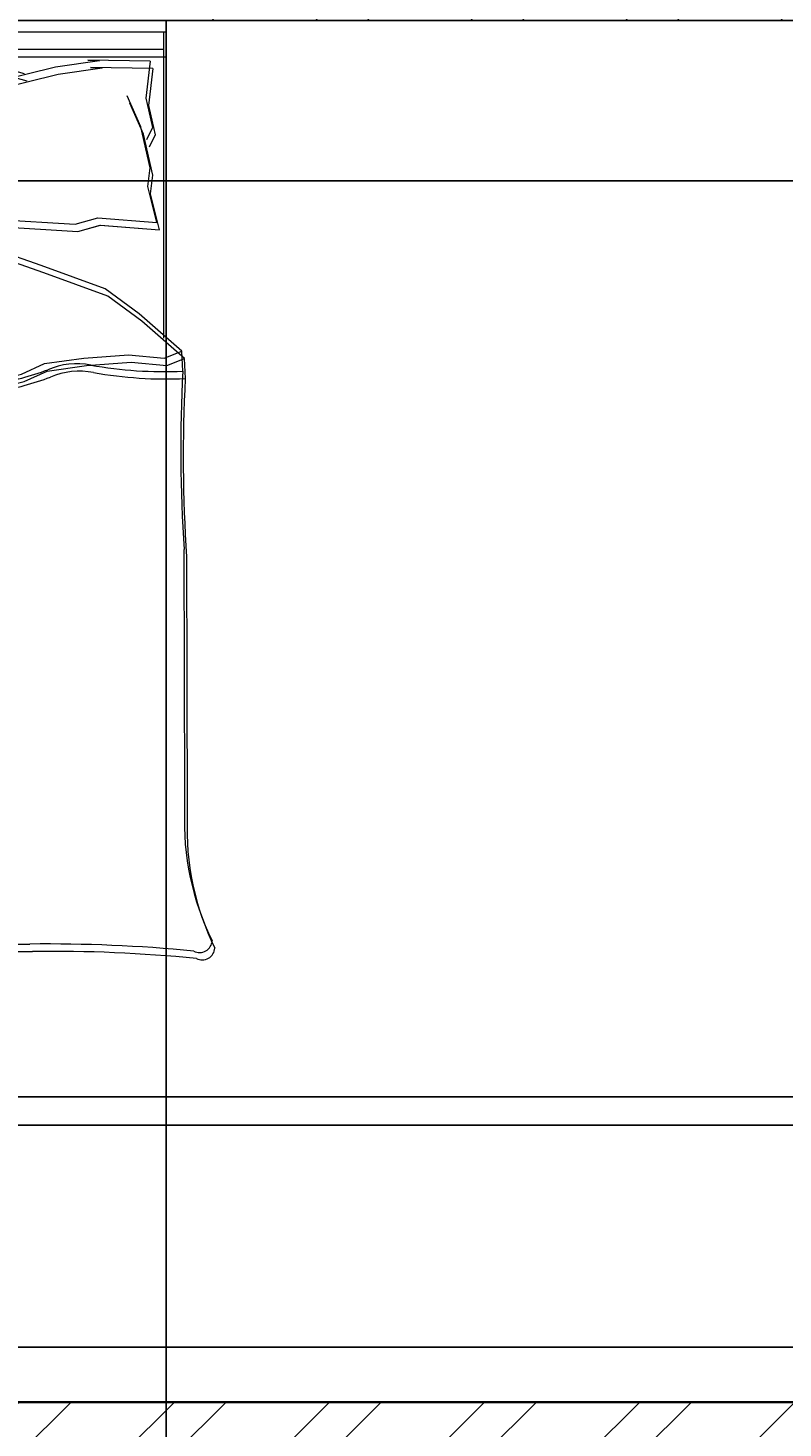
# Model space of a CAD drawing. Units: inches. Extents: x 1748 to 2382, y 1346 to 2284.
# Tile 22 of 26: x 1956 to 2022, y 2102 to 2223. Entities that reach past the tile are written whole.
import ezdxf

# ---------------------------------------------------------------- set-up
doc = ezdxf.new("R2010")
doc.units = ezdxf.units.IN
for name, color, linetype, lineweight in [('A-ANNO-DIMS', 2, 'Continuous', 18), ('A-FURN', 8, 'Continuous', 13), ('A-WALL', 7, 'Continuous', 35), ('A-WALL-PATT', 9, 'Continuous', 13)]:
    doc.layers.add(name, color=color, linetype=linetype, lineweight=lineweight)
doc.styles.get("Standard").update_dxf_attribs({"font": 'arial.ttf'})
doc.dimstyles.get("Standard").update_dxf_attribs({"dimtxt": 0.18, "dimasz": 0.18, "dimexe": 0.18, "dimexo": 0.0625, "dimgap": 0.09, "dimtad": 0, "dimtih": 1, "dimtoh": 1, "dimdec": 4, "dimzin": 0, "dimdsep": 46, "dimtxsty": 'Standard', "dimcen": 0.09, "dimadec": 0, "dimazin": 0, "dimtfac": 1, "dimtdec": 4, "dimtofl": 0, "dimtmove": 0, "dimatfit": 3, "dimfxl": 1, "dimtolj": 1, "dimtzin": 0, "dimarcsym": 0})

# ---------------------------------------------------------------- blocks, each defined once
blk = doc.blocks.new('BED-DOUBLE')
for p, q in [((3.48, 63.33), (3.48, 81.44)), ((3.48, 63.33), (3.48, 81.44)), ((3.48, 81.44), (51.49, 81.44)), ((3.7, 62.69), (3.7, 80.8)), ((3.7, 62.69), (3.7, 80.8)), ((51.27, 81.44), (51.27, 54.83)), ((51.27, 81.44), (51.27, 54.83)), ((51.49, 81.44), (51.49, 80.8)), ((51.49, 80.8), (51.49, 54.19)), ((51.49, 80.8), (51.49, 54.19)), ((3.48, 79.91), (51.27, 79.91)), ((3.48, 79.91), (51.27, 79.91)), ((3.7, 79.27), (51.49, 79.27)), ((3.7, 79.27), (51.49, 79.27)), ((16.88, 78.42), (19.77, 79.14)), ((16.88, 78.42), (19.77, 79.14)), ((19.77, 79.14), (20.09, 79.14)), ((19.77, 79.14), (20.09, 79.14)), ((20.09, 79.14), (24.54, 78.99)), ((20.09, 79.14), (24.54, 78.99)), ((24.54, 78.99), (25.98, 79.57)), ((24.54, 78.99), (25.98, 79.57)), ((25.98, 79.57), (26.56, 74.22)), ((25.98, 79.57), (26.56, 74.22)), ((3.89, 78.13), (4.47, 74.95)), ((3.9, 78.11), (8.18, 78.43)), ((3.9, 78.11), (8.18, 78.43)), ((3.9, 78.13), (4.47, 74.95)), ((8.18, 78.43), (8.29, 78.42)), ((8.18, 78.43), (8.28, 78.42)), ((8.28, 78.42), (12.11, 78.13)), ((8.29, 78.42), (12.11, 78.13)), ((12.11, 78.13), (17.6, 77.12)), ((12.11, 78.13), (17.6, 77.12)), ((14.86, 77.69), (16.88, 78.42)), ((14.86, 77.69), (16.88, 78.42)), ((17.11, 77.78), (20, 78.5)), ((17.11, 77.78), (20, 78.5)), ((20, 78.5), (20.32, 78.5)), ((20, 78.5), (20.32, 78.5)), ((20.32, 78.5), (24.77, 78.36)), ((20.32, 78.5), (24.77, 78.36)), ((24.77, 78.36), (26.21, 78.93)), ((24.77, 78.36), (26.21, 78.93)), ((26.21, 78.93), (26.79, 73.58)), ((26.21, 78.93), (26.79, 73.58)), ((27.98, 78.95), (27.73, 73.58)), ((27.98, 78.95), (27.73, 73.58)), ((28.21, 78.31), (27.96, 72.94)), ((28.21, 78.31), (27.96, 72.94)), ((29.46, 78.46), (27.98, 78.95)), ((29.46, 78.46), (27.98, 78.95)), ((29.68, 77.83), (28.21, 78.31)), ((29.68, 77.83), (28.21, 78.31)), ((33.88, 78.89), (29.46, 78.46)), ((33.88, 78.89), (29.46, 78.46)), ((34.11, 78.25), (29.68, 77.83)), ((34.11, 78.25), (29.68, 77.83)), ((34.21, 78.91), (33.88, 78.89)), ((34.2, 78.91), (33.88, 78.89)), ((34.43, 78.27), (34.11, 78.25)), ((34.43, 78.27), (34.11, 78.25)), ((37.14, 78.37), (34.2, 78.91)), ((37.14, 78.37), (34.21, 78.91)), ((37.36, 77.73), (34.43, 78.27)), ((37.36, 77.73), (34.43, 78.27)), ((41.91, 78.37), (36.5, 77.02)), ((41.91, 78.37), (36.5, 77.02)), ((39.2, 77.77), (37.14, 78.37)), ((39.2, 77.77), (37.14, 78.37)), ((45.71, 78.9), (41.91, 78.37)), ((45.71, 78.9), (41.91, 78.37)), ((45.94, 78.26), (42.14, 77.73)), ((45.94, 78.26), (42.14, 77.73)), ((50.11, 78.89), (44.71, 78.98)), ((44.71, 78.98), (45.71, 78.9)), ((50.11, 78.89), (44.71, 78.98)), ((44.71, 78.98), (45.71, 78.9)), ((50.34, 78.25), (44.94, 78.34)), ((44.94, 78.34), (45.94, 78.26)), ((50.34, 78.25), (44.94, 78.34)), ((44.94, 78.34), (45.94, 78.26)), ((50.11, 78.89), (49.73, 75.68)), ((50.11, 78.89), (49.73, 75.68)), ((50.34, 78.25), (49.96, 75.04)), ((50.34, 78.25), (49.96, 75.04)), ((4.12, 77.49), (4.7, 74.31)), ((4.12, 77.49), (4.7, 74.31)), ((4.13, 77.47), (8.41, 77.8)), ((4.13, 77.47), (8.41, 77.8)), ((8.41, 77.8), (8.51, 77.78)), ((8.41, 77.8), (8.51, 77.78)), ((8.51, 77.78), (12.34, 77.49)), ((8.51, 77.78), (12.34, 77.49)), ((12.34, 77.49), (17.83, 76.48)), ((12.34, 77.49), (17.83, 76.48)), ((15.08, 77.05), (17.11, 77.78)), ((15.08, 77.05), (17.11, 77.78)), ((42.14, 77.73), (36.72, 76.38)), ((42.14, 77.73), (36.72, 76.38)), ((39.43, 77.13), (37.36, 77.73)), ((39.43, 77.13), (37.36, 77.73)), ((49.31, 73.19), (48.13, 75.87)), ((49.31, 73.19), (48.13, 75.87)), ((49.73, 75.68), (50.33, 73.11)), ((49.73, 75.68), (50.33, 73.11)), ((4.47, 74.95), (4.04, 72.34)), ((4.47, 74.95), (4.04, 72.34)), ((4.7, 74.31), (4.27, 71.7)), ((4.7, 74.31), (4.27, 71.7)), ((5.05, 72.49), (6.06, 75.24)), ((5.05, 72.49), (6.06, 75.24)), ((5.28, 71.85), (6.29, 74.6)), ((5.28, 71.85), (6.29, 74.6)), ((26.56, 74.22), (27.14, 71.04)), ((26.56, 74.22), (27.14, 71.04)), ((49.54, 72.55), (48.36, 75.23)), ((49.54, 72.55), (48.36, 75.23)), ((49.96, 75.04), (50.56, 72.47)), ((49.96, 75.04), (50.56, 72.47)), ((26.79, 73.58), (27.37, 70.4)), ((26.79, 73.58), (27.37, 70.4)), ((27.73, 73.58), (27.35, 70.37)), ((27.73, 73.58), (27.36, 70.37)), ((50.11, 69.61), (49.31, 73.19)), ((50.11, 69.61), (49.31, 73.19)), ((50.33, 73.11), (49.81, 72.06)), ((50.33, 73.11), (49.81, 72.06)), ((4.04, 72.34), (4.62, 71.33)), ((4.04, 72.34), (4.62, 71.33)), ((4.47, 68.87), (5.05, 72.49)), ((4.47, 68.87), (5.05, 72.49)), ((4.7, 68.23), (5.28, 71.85)), ((4.7, 68.23), (5.28, 71.85)), ((27.96, 72.94), (27.58, 69.73)), ((27.96, 72.94), (27.58, 69.73)), ((50.34, 68.98), (49.54, 72.55)), ((50.34, 68.98), (49.54, 72.55)), ((50.56, 72.47), (50.04, 71.42)), ((50.56, 72.47), (50.04, 71.42)), ((4.27, 71.7), (4.85, 70.69)), ((4.27, 71.7), (4.85, 70.69)), ((27.14, 71.04), (27.14, 69.74)), ((27.14, 71.04), (27.14, 69.74)), ((27.14, 69.74), (26.56, 67.86)), ((27.14, 69.74), (26.56, 67.86)), ((27.35, 70.37), (27.44, 69.07)), ((27.36, 70.37), (27.44, 69.07)), ((27.37, 70.4), (27.37, 69.1)), ((27.37, 70.4), (27.37, 69.1)), ((27.58, 69.73), (27.66, 68.43)), ((27.58, 69.73), (27.66, 68.43)), ((49.92, 68.01), (50.11, 69.61)), ((49.92, 68.01), (50.11, 69.61)), ((4.76, 67.28), (4.47, 68.87)), ((4.76, 67.28), (4.47, 68.87)), ((4.99, 66.64), (4.7, 68.23)), ((4.99, 66.64), (4.7, 68.23)), ((27.37, 69.1), (26.79, 67.22)), ((27.37, 69.1), (26.79, 67.22)), ((27.44, 69.07), (28.13, 67.23)), ((27.44, 69.07), (28.13, 67.23)), ((27.66, 68.43), (28.36, 66.59)), ((27.66, 68.43), (28.36, 66.59)), ((50.15, 67.37), (50.34, 68.98)), ((50.15, 67.37), (50.34, 68.98)), ((4.18, 64.1), (4.76, 67.28)), ((4.18, 64.1), (4.76, 67.28)), ((26.56, 67.86), (26.56, 65.18)), ((26.56, 67.86), (26.56, 65.18)), ((26.79, 67.22), (26.79, 64.54)), ((26.79, 67.22), (26.79, 64.54)), ((28.13, 67.23), (28.3, 64.55)), ((28.13, 67.23), (28.3, 64.55)), ((50.7, 64.87), (49.92, 68.01)), ((50.7, 64.87), (49.92, 68.01)), ((50.93, 64.23), (50.15, 67.37)), ((50.93, 64.23), (50.15, 67.37)), ((4.41, 63.46), (4.99, 66.64)), ((4.41, 63.46), (4.99, 66.64)), ((6.38, 65.81), (10.41, 65.15)), ((6.38, 65.81), (10.41, 65.15)), ((24.1, 65.18), (20.96, 66.27)), ((24.1, 65.18), (20.96, 66.27)), ((28.36, 66.59), (28.53, 63.91)), ((28.36, 66.59), (28.53, 63.91)), ((30.75, 64.7), (33.82, 65.99)), ((30.75, 64.7), (33.82, 65.99)), ((32.56, 65.81), (36.6, 65.15)), ((32.56, 65.81), (36.6, 65.15)), ((9.28, 64.83), (4.18, 64.1)), ((9.28, 64.83), (4.18, 64.1)), ((6.61, 65.18), (10.64, 64.51)), ((6.61, 65.18), (10.64, 64.51)), ((10.41, 65.15), (9.28, 64.83)), ((10.41, 65.15), (9.28, 64.83)), ((10.64, 64.51), (9.51, 64.19)), ((10.64, 64.51), (9.51, 64.19)), ((10.41, 65.15), (17.42, 64.72)), ((10.41, 65.15), (17.42, 64.72)), ((10.64, 64.51), (17.65, 64.08)), ((10.64, 64.51), (17.65, 64.08)), ((17.42, 64.72), (19.38, 65.27)), ((17.42, 64.72), (19.38, 65.27)), ((17.65, 64.08), (19.61, 64.64)), ((17.65, 64.08), (19.61, 64.64)), ((19.38, 65.27), (24.52, 64.87)), ((19.38, 65.27), (24.52, 64.87)), ((19.61, 64.64), (24.74, 64.23)), ((19.61, 64.64), (24.74, 64.23)), ((24.33, 64.54), (21.19, 65.63)), ((24.33, 64.54), (21.19, 65.63)), ((26.56, 65.18), (24.1, 65.18)), ((26.56, 65.18), (24.1, 65.18)), ((26.79, 64.54), (24.33, 64.54)), ((26.79, 64.54), (24.33, 64.54)), ((28.3, 64.55), (30.75, 64.7)), ((28.3, 64.55), (30.75, 64.7)), ((30.98, 64.06), (34.05, 65.35)), ((30.98, 64.06), (34.05, 65.35)), ((32.79, 65.18), (36.83, 64.51)), ((32.79, 65.18), (36.82, 64.51)), ((36.6, 65.15), (43.61, 64.72)), ((36.6, 65.15), (43.61, 64.72)), ((36.82, 64.51), (43.83, 64.08)), ((36.83, 64.51), (43.83, 64.08)), ((43.61, 64.72), (45.57, 65.27)), ((43.61, 64.72), (45.57, 65.27)), ((43.83, 64.08), (45.8, 64.64)), ((43.83, 64.08), (45.79, 64.64)), ((45.57, 65.27), (50.7, 64.87)), ((45.57, 65.27), (50.7, 64.87)), ((45.79, 64.64), (50.93, 64.23)), ((45.8, 64.64), (50.93, 64.23)), ((9.51, 64.19), (4.41, 63.46)), ((9.51, 64.19), (4.41, 63.46)), ((28.53, 63.91), (30.98, 64.06)), ((28.53, 63.91), (30.98, 64.06)), ((30.26, 64.06), (34.45, 57.57)), ((30.26, 64.06), (34.45, 57.57)), ((30.49, 63.42), (34.68, 56.93)), ((30.49, 63.42), (34.68, 56.93)), ((40.64, 61.13), (32.31, 64.06)), ((40.64, 61.13), (32.31, 64.06)), ((40.87, 60.49), (32.53, 63.42)), ((40.87, 60.49), (32.53, 63.42)), ((46.22, 59.11), (40.64, 61.13)), ((46.22, 59.11), (40.64, 61.13)), ((46.45, 58.48), (40.87, 60.49)), ((46.45, 58.48), (40.87, 60.49)), ((49.16, 56.95), (46.22, 59.11)), ((49.16, 56.95), (46.22, 59.11)), ((49.39, 56.31), (46.45, 58.48)), ((49.39, 56.31), (46.45, 58.48)), ((34.45, 57.57), (36.15, 53.08)), ((34.45, 57.57), (36.15, 53.08)), ((34.68, 56.93), (36.38, 52.44)), ((34.68, 56.93), (36.38, 52.44)), ((52.87, 53.7), (49.16, 56.95)), ((52.87, 53.7), (49.16, 56.95)), ((53.1, 53.06), (49.39, 56.31)), ((53.1, 53.06), (49.39, 56.31)), ((51.33, 53.08), (52.87, 53.7)), ((51.33, 53.08), (52.87, 53.7)), ((52.95, 51.95), (52.87, 53.7, 3.87)), ((52.95, 51.95), (52.87, 53.7, 3.87)), ((36.15, 53.08), (36.46, 51.07)), ((36.15, 53.08), (36.46, 51.07)), ((36.38, 52.44), (36.69, 50.43)), ((36.38, 52.44), (36.69, 50.43)), ((38.94, 51.69), (40.95, 52.61)), ((38.94, 51.69), (40.95, 52.61)), ((40.95, 52.61), (44.36, 53.08)), ((40.95, 52.61), (44.36, 53.08)), ((41.18, 51.97), (44.59, 52.44)), ((41.18, 51.97), (44.59, 52.44)), ((44.36, 53.08), (48.23, 53.39)), ((44.36, 53.08), (48.23, 53.39)), ((44.59, 52.44), (48.46, 52.75)), ((44.59, 52.44), (48.46, 52.75)), ((48.23, 53.39), (51.33, 53.08)), ((48.23, 53.39), (51.33, 53.08)), ((48.46, 52.75), (51.56, 52.44)), ((48.46, 52.75), (51.56, 52.44)), ((51.56, 52.44), (53.1, 53.06)), ((51.56, 52.44), (53.1, 53.06)), ((53.18, 51.31), (53.1, 53.06, 3.87)), ((53.18, 51.31), (53.1, 53.06, 3.87)), ((36.46, 51.07), (38.94, 51.69)), ((36.46, 51.07), (38.94, 51.69)), ((39.17, 51.05), (41.18, 51.97)), ((39.17, 51.05), (41.18, 51.97)), ((36.69, 50.43), (39.17, 51.05)), ((36.69, 50.43), (39.17, 51.05)), ((15.06, 2.2), (39.68, 2.2)), ((15.06, 2.2), (39.68, 2.2)), ((15.29, 1.56), (39.91, 1.56)), ((15.29, 1.56), (39.91, 1.56))]:
    blk.add_line(p, q)
for centre, radius, start, end in [((21.36, -100.61), 164.97, 86.0865, 96.7821), ((21.36, -100.61), 164.97, 86.0865, 96.7821), ((21.59, -101.25), 164.97, 86.0865, 96.7821), ((21.59, -101.25), 164.97, 86.0865, 96.7821), ((85.16, 61.35), 83.31, 178.7218, 185.604), ((85.16, 61.35), 83.31, 178.7218, 185.604), ((85.39, 60.71), 83.31, 178.7218, 185.604), ((85.39, 60.71), 83.31, 178.7218, 185.604), ((17.76, -74.87), 129.02, 81.7845, 96.9006), ((17.76, -74.87), 129.02, 81.7845, 96.9006), ((17.98, -75.51), 129.02, 81.7845, 96.9006), ((17.98, -75.51), 129.02, 81.7845, 96.9006), ((-167.31, 50.27), 170.11, 358.4762, 1.0082), ((-167.31, 50.27), 170.11, 358.4762, 1.0082), ((-167.08, 49.63), 170.11, 358.4762, 1.0082), ((-167.08, 49.63), 170.11, 358.4762, 1.0082), ((43.74, 46.38), 6.22, 78.6608, 113.7384), ((43.74, 46.38), 6.22, 78.6608, 113.7384), ((51.33, 88.1), 36.18, 259.8763, 272.5657), ((51.33, 88.1), 36.18, 259.8763, 272.5657), ((31.15, 79.96), 29.65, 280.6617, 289.8806), ((31.15, 79.96), 29.65, 280.6617, 289.8806), ((31.38, 79.32), 29.65, 280.6617, 289.8806), ((31.38, 79.32), 29.65, 280.6617, 289.8806), ((43.97, 45.74), 6.22, 78.6608, 113.7384), ((43.97, 45.74), 6.22, 78.6608, 113.7384), ((51.56, 87.46), 36.18, 259.8763, 272.5657), ((51.56, 87.46), 36.18, 259.8763, 272.5657), ((182.27, 45.13), 129.5, 176.9791, 183.8365), ((182.27, 45.13), 129.5, 176.9791, 183.8365), ((182.49, 44.49), 129.5, 176.9791, 183.8365), ((182.49, 44.49), 129.5, 176.9791, 183.8365), ((36.64, 51), 0.185, 160.2464, 271.1377), ((36.64, 51), 0.185, 160.2464, 271.1377), ((36.87, 50.36), 0.185, 160.2464, 271.1377), ((36.86, 50.36), 0.185, 160.2464, 271.1377), ((484.82, 30.83), 482.31, 178.2277, 181.7185), ((484.82, 30.83), 482.31, 178.2277, 181.7185), ((485.05, 30.19), 482.31, 178.2277, 181.7185), ((485.05, 30.19), 482.31, 178.2277, 181.7185), ((-4508.74, 13.62), 4561.86, 0.00217, 0.28689), ((-4508.74, 13.62), 4561.86, 0.00217, 0.28689), ((-4508.51, 12.98), 4561.86, 0.00217, 0.28689), ((-4508.51, 12.98), 4561.86, 0.00217, 0.28689), ((-26.9, 16.93), 29.63, 346.0648, 358.9113), ((-26.9, 16.93), 29.63, 346.0648, 358.9113), ((-26.67, 16.29), 29.63, 346.0648, 358.9113), ((-26.67, 16.29), 29.63, 346.0648, 358.9113), ((76.16, 12.78), 23.07, 177.4714, 206.4681), ((76.16, 12.78), 23.07, 177.4714, 206.4681), ((76.39, 12.14), 23.07, 177.4714, 206.4681), ((76.39, 12.14), 23.07, 177.4714, 206.4681), ((-21.66, 11.17), 23.56, 337.9751, 356.652), ((-21.66, 11.17), 23.56, 337.9751, 356.652), ((-21.43, 10.53), 23.56, 337.9751, 356.652), ((-21.43, 10.53), 23.56, 337.9751, 356.652), ((-17.22, 105.16), 106.46, 283.3832, 287.7053), ((-17.22, 105.16), 106.46, 283.3832, 287.7053), ((-16.99, 104.52), 106.46, 283.3832, 287.7053), ((-16.99, 104.52), 106.46, 283.3832, 287.7053), ((54.41, 2.57), 1.1, 242.6588, 356.02), ((54.41, 2.57), 1.1, 242.6588, 356.02), ((1.09, 1.73), 1.09, 146.1736, 293.4781), ((1.09, 1.73), 1.09, 146.1736, 293.4781), ((1.32, 1.09), 1.09, 146.1736, 293.4781), ((1.32, 1.09), 1.09, 146.1736, 293.4781), ((21.43, -119.39), 121.76, 92.9958, 99.4091), ((21.43, -119.39), 121.76, 92.9958, 99.4091), ((21.66, -120.03), 121.76, 92.9958, 99.4091), ((21.66, -120.03), 121.76, 92.9958, 99.4091), ((41.15, -130.83), 133.04, 84.4998, 90.6351), ((41.15, -130.83), 133.04, 84.4998, 90.6351), ((41.38, -131.47), 133.04, 84.4998, 90.6351), ((41.38, -131.47), 133.04, 84.4998, 90.6351), ((54.64, 1.93), 1.1, 242.6588, 356.02), ((54.64, 1.93), 1.1, 242.6588, 356.02)]:
    blk.add_arc(centre, radius, start, end)
blk = doc.blocks.new('*D51')
at = {"layer": 'A-ANNO-DIMS', "color": 0, "lineweight": -2, "transparency": 16777216}
for p, q in [((1968.44, 2223.79), (1968.44, 1360.47)), ((2040.07, 2223.79), (2040.07, 1360.47)), ((1968.62, 1360.65), (2003.86, 1360.65)), ((2039.89, 1360.65), (2004.65, 1360.65))]:
    blk.add_line(p, q, dxfattribs=at)
at = {"layer": 'A-ANNO-DIMS', "color": 0, "transparency": 16777216}
for points in [[(1968.62, 1360.68), (1968.62, 1360.62), (1968.44, 1360.65)], [(2039.89, 1360.68), (2039.89, 1360.62), (2040.07, 1360.65)]]:
    blk.add_solid(points, dxfattribs=at)
at = {"layer": 'Defpoints', "color": 0, "transparency": 16777216}
for p in [(1968.44, 2223.85), (2040.07, 2223.85), (2040.07, 1360.65)]:
    blk.add_point(p, dxfattribs=at)
at = {"layer": 'A-ANNO-DIMS', "color": 0, "transparency": 16777216, "insert": (2004.26, 1360.65), "char_height": 0.18, "attachment_point": 5}
blk.add_mtext('\\A1;71.62', dxfattribs=at)
blk = doc.blocks.new('*D68')
at = {"layer": 'A-ANNO-DIMS', "color": 0, "lineweight": -2, "transparency": 16777216}
for p, q in [((1865.52, 2223.85), (2339.54, 2223.85)), ((2339.36, 2223.67), (2339.36, 2217.07)), ((2339.36, 2210.1), (2339.36, 2216.7)), ((1865.52, 2209.92), (2339.54, 2209.92))]:
    blk.add_line(p, q, dxfattribs=at)
at = {"layer": 'A-ANNO-DIMS', "color": 0, "transparency": 16777216}
for points in [[(2339.33, 2223.67), (2339.39, 2223.67), (2339.36, 2223.85)], [(2339.33, 2210.1), (2339.39, 2210.1), (2339.36, 2209.92)]]:
    blk.add_solid(points, dxfattribs=at)
at = {"layer": 'Defpoints', "color": 0, "transparency": 16777216}
for p in [(1865.46, 2223.85), (2339.36, 2223.85), (1865.46, 2209.92)]:
    blk.add_point(p, dxfattribs=at)
at = {"layer": 'A-ANNO-DIMS', "color": 0, "transparency": 16777216, "insert": (2339.36, 2216.88), "char_height": 0.18, "attachment_point": 5}
blk.add_mtext('\\A1;13.93', dxfattribs=at)
blk = doc.blocks.new('*D75')
at = {"layer": 'A-ANNO-DIMS', "color": 0, "lineweight": -2, "transparency": 16777216}
for p, q in [((2078.4, 2130.35), (1779.88, 2130.35)), ((1780.06, 2130.17), (1780.06, 2117.28)), ((1780.06, 2104.03), (1780.06, 2116.92)), ((2078.4, 2103.85), (1779.88, 2103.85))]:
    blk.add_line(p, q, dxfattribs=at)
at = {"layer": 'A-ANNO-DIMS', "color": 0, "transparency": 16777216}
for points in [[(1780.03, 2130.17), (1780.09, 2130.17), (1780.06, 2130.35)], [(1780.03, 2104.03), (1780.09, 2104.03), (1780.06, 2103.85)]]:
    blk.add_solid(points, dxfattribs=at)
at = {"layer": 'Defpoints', "color": 0, "transparency": 16777216}
for p in [(1780.06, 2130.35), (2078.46, 2130.35), (2078.46, 2103.85)]:
    blk.add_point(p, dxfattribs=at)
at = {"layer": 'A-ANNO-DIMS', "color": 0, "transparency": 16777216, "insert": (1780.06, 2117.1), "char_height": 0.18, "attachment_point": 5}
blk.add_mtext('\\A1;26.5', dxfattribs=at)
blk = doc.blocks.new('*D77')
at = {"layer": 'A-ANNO-DIMS', "color": 0, "lineweight": -2, "transparency": 16777216}
for p, q in [((1870.02, 2127.89), (2339.54, 2127.89)), ((2339.36, 2127.71), (2339.36, 2118.43)), ((2339.36, 2108.79), (2339.36, 2118.07)), ((1870.02, 2108.61), (2339.54, 2108.61))]:
    blk.add_line(p, q, dxfattribs=at)
at = {"layer": 'A-ANNO-DIMS', "color": 0, "transparency": 16777216}
for points in [[(2339.33, 2127.71), (2339.39, 2127.71), (2339.36, 2127.89)], [(2339.33, 2108.79), (2339.39, 2108.79), (2339.36, 2108.61)]]:
    blk.add_solid(points, dxfattribs=at)
at = {"layer": 'Defpoints', "color": 0, "transparency": 16777216}
for p in [(1869.96, 2127.89), (2339.36, 2127.89), (1869.96, 2108.61)]:
    blk.add_point(p, dxfattribs=at)
at = {"layer": 'A-ANNO-DIMS', "color": 0, "transparency": 16777216, "insert": (2339.36, 2118.25), "char_height": 0.18, "attachment_point": 5}
blk.add_mtext('\\A1;19.288', dxfattribs=at)

msp = doc.modelspace()

# ---------------------------------------------------------------- hatches: boundary and pattern name
at = {"layer": 'A-WALL-PATT'}
h = msp.add_hatch(dxfattribs=at)
h.set_pattern_fill('ANSI32', color=256)
h.paths.add_polyline_path([(1908.4445, 2232.8497), (1821.9607, 2232.8497), (1821.9607, 2223.8497), (1865.4607, 2223.8497), (1865.4607, 2209.9185), (1869.9607, 2209.9185), (1869.9607, 2223.8497), (1908.4445, 2223.8497), (1908.4445, 2228.3497)])
h.paths.add_polyline_path([(2040.0683, 2232.8497), (1968.4445, 2232.8497), (1968.4445, 2223.8497), (2025.9607, 2223.8497), (2025.9607, 2130.3497), (2032.1341, 2130.3497), (2032.1341, 2132.5997), (2032.1341, 2134.8497), (2030.4607, 2134.8497), (2030.4607, 2223.8497), (2040.0683, 2223.8497)])
h.paths.add_polyline_path([(2091.3969, 2232.8497), (2064.0683, 2232.8497), (2064.0683, 2223.8497), (2078.4607, 2223.8497), (2078.4607, 2134.8497), (2051.1563, 2134.8497), (2051.1563, 2130.3497), (2078.4607, 2130.3497), (2078.4607, 2128.6813), (2082.9607, 2128.6813), (2082.9607, 2130.3497), (2086.1879, 2130.3497), (2086.1879, 2132.5997), (2086.1879, 2134.8497), (2082.9607, 2134.8497), (2082.9607, 2223.8497), (2091.3969, 2223.8497), (2091.3969, 2228.3497)])
h.paths.add_polyline_path([(2167.0164, 2232.8497), (2115.3969, 2232.8497), (2115.3969, 2223.8497), (2130.9607, 2223.8497), (2130.9607, 2134.8497), (2106.9607, 2134.8497), (2106.9607, 2130.3497), (2135.4607, 2130.3497), (2135.4607, 2223.8497), (2167.0164, 2223.8497), (2167.0164, 2228.3497)])
h.paths.add_polyline_path([(1869.9607, 2149.9185), (1865.4607, 2149.9185), (1865.4607, 2127.8942), (1869.9607, 2127.8942)])
h.paths.add_polyline_path([(2082.9607, 2104.4871), (2080.7107, 2104.4871), (2078.4607, 2104.4871), (2078.4607, 2103.8497), (1869.9607, 2103.8497), (1869.9607, 2108.6062), (1867.7107, 2108.6062), (1865.4607, 2108.6062), (1865.4607, 2103.8497), (1821.9607, 2103.8497), (1821.9607, 2099.3497), (1865.4607, 2099.3497), (1865.4607, 2094.7509), (1869.9607, 2094.7509), (1869.9607, 2099.3497), (2025.9607, 2099.3497), (2025.9607, 2096.4326), (2030.4607, 2096.4326), (2030.4607, 2099.3497), (2082.9607, 2099.3497)])
h.paths.add_polyline_path([(1928.9457, 1401.1212), (2176.8693, 1401.1212), (2176.8693, 1438.214), (1928.9457, 1438.214)], flags=9)
h.paths.add_polyline_path([(2122.2668, 2048.1927), (2177.9387, 2048.1927), (2177.9387, 2066.85), (2122.2668, 2066.85)], flags=9)
h.paths.add_polyline_path([(2272.688, 2153.8197), (2272.688, 2216.746), (2262.3845, 2216.746), (2262.3845, 2153.8197)], flags=9)
h.paths.add_polyline_path([(2157.2928, 2166.5593), (2196.3822, 2166.5593), (2196.3822, 2185.2167), (2157.2928, 2185.2167)], flags=9)
h.paths.add_polyline_path([(2089.3407, 2162.0698), (2124.3987, 2162.0698), (2124.3987, 2180.7272), (2089.3407, 2180.7272)], flags=9)
h.paths.add_polyline_path([(2037.4521, 2160.0913), (2072.5101, 2160.0913), (2072.5101, 2178.7486), (2037.4521, 2178.7486)], flags=9)
h.paths.add_polyline_path([(1884.7894, 2104.1554), (1923.6297, 2104.1554), (1923.6297, 2122.8127), (1884.7894, 2122.8127)], flags=9)
h.paths.add_polyline_path([(1851.2832, 2142.9749), (1851.2832, 2199.3051), (1840.9796, 2199.3051), (1840.9796, 2142.9749)], flags=9)
h.paths.add_polyline_path([(1844.8763, 2017.2834), (1844.8763, 2073.6136), (1834.5728, 2073.6136), (1834.5728, 2017.2834)], flags=9)
h.paths.add_polyline_path([(1897.1577, 2073.1279), (1935.9981, 2073.1279), (1935.9981, 2091.7853), (1897.1577, 2091.7853)], flags=9)
h.paths.add_polyline_path([(1952.3395, 1802.4231), (2008.0114, 1802.4231), (2008.0114, 1821.0805), (1952.3395, 1821.0805)], flags=9)
h.paths.add_polyline_path([(1978.8184, 1857.6841), (2017.7338, 1857.6841), (2017.7338, 1876.3415), (1978.8184, 1876.3415)], flags=9)
h.paths.add_polyline_path([(1979.6513, 1925.9516), (2008.8089, 1925.9516), (2008.8089, 1944.6089), (1979.6513, 1944.6089)], flags=9)
h.paths.add_polyline_path([(1838.5553, 1860.3527), (1877.3957, 1860.3527), (1877.3957, 1879.01), (1838.5553, 1879.01)], flags=9)
h.paths.add_polyline_path([(1883.9018, 1787.3013), (1883.9018, 1843.6315), (1873.5983, 1843.6315), (1873.5983, 1787.3013)], flags=9)
h.paths.add_polyline_path([(1873.7079, 1509.1938), (1873.7079, 1583.7709), (1863.4044, 1583.7709), (1863.4044, 1509.1938)], flags=9)
h.paths.add_polyline_path([(1916.2259, 1603.3681), (1955.0663, 1603.3681), (1955.0663, 1622.0254), (1916.2259, 1622.0254)], flags=9)
h.paths.add_polyline_path([(1876.3013, 1636.757), (1876.3013, 1693.0871), (1865.9978, 1693.0871), (1865.9978, 1636.757)], flags=9)
h.paths.add_polyline_path([(1921.3138, 1521.8316), (1964.0662, 1521.8316), (1964.0662, 1540.489), (1921.3138, 1540.489)], flags=9)
h.paths.add_polyline_path([(2017.5657, 1497.5078), (2046.7983, 1497.5078), (2046.7983, 1516.1651), (2017.5657, 1516.1651)], flags=9)
h.paths.add_polyline_path([(2066.8661, 1499.3902), (2096.0988, 1499.3902), (2096.0988, 1518.0475), (2066.8661, 1518.0475)], flags=9)
h.paths.add_polyline_path([(2155.4835, 1571.6596), (2198.2358, 1571.6596), (2198.2358, 1590.3169), (2155.4835, 1590.3169)], flags=9)
h.paths.add_polyline_path([(2094.9136, 1664.6812), (2150.5855, 1664.6812), (2150.5855, 1683.3386), (2094.9136, 1683.3386)], flags=9)
h.paths.add_polyline_path([(2257.6902, 1863.1628), (2269.8935, 1863.1628), (2269.8935, 1873.4664), (2257.6902, 1873.4664)], flags=9)
h.paths.add_polyline_path([(2164.0748, 1880.3089), (2189.8694, 1880.3089), (2189.8694, 1890.6124), (2164.0748, 1890.6124)], flags=9)
h.paths.add_polyline_path([(2239.4394, 1931.0585), (2268.8187, 1931.0585), (2268.8187, 1949.7159), (2239.4394, 1949.7159)], flags=9)

# ---------------------------------------------------------------- linework, layer by layer
at = {"layer": 'A-WALL'}
msp.add_line((1869.9607, 2103.8497), (2078.4607, 2103.8497), dxfattribs=at)

# ---------------------------------------------------------------- block references
at = {"layer": 'A-FURN'}
msp.add_blockref('BED-DOUBLE', (1916.92, 2141.426), dxfattribs=at)

# ---------------------------------------------------------------- dimensions: what is measured, and where the dimension line sits
at = {"layer": 'A-ANNO-DIMS'}
for base, p1, p2, override, picture, middle in [((2339.3607, 2223.8497), (1865.4607, 2209.9185), (1865.4607, 2223.8497), {"dimdec": 2, "dimlfac": 1, "dimrnd": 0, "dimzin": 0, "dimdsep": 46, "dimlunit": 2}, '*D68', (2339.3607, 2216.8841)), ((1780.0607, 2130.3497), (2078.4607, 2103.8497), (2078.4607, 2130.3497), {"dimdec": 1, "dimlfac": 1, "dimrnd": 0, "dimzin": 0, "dimdsep": 46, "dimlunit": 2}, '*D75', (1780.0607, 2117.0997)), ((2339.3607, 2127.8942), (1869.9607, 2108.6062), (1869.9607, 2127.8942), {"dimdec": 3, "dimlfac": 1, "dimrnd": 0, "dimzin": 0, "dimdsep": 46, "dimlunit": 2}, '*D77', (2339.3607, 2118.2502))]:
    dim = msp.add_linear_dim(base=base, p1=p1, p2=p2, angle=90, dimstyle='Standard', override=override, dxfattribs=at)
    dim.commit()
    dim.dimension.update_dxf_attribs({"geometry": picture, "text_midpoint": middle})
dim = msp.add_linear_dim(base=(2040.0683, 1360.6451), p1=(1968.4445, 2223.8497), p2=(2040.0683, 2223.8497), dimstyle='Standard', override={"dimdec": 2, "dimlfac": 1, "dimrnd": 0, "dimzin": 0, "dimdsep": 46, "dimlunit": 2}, dxfattribs=at)
dim.commit()
dim.dimension.update_dxf_attribs({"geometry": '*D51', "text_midpoint": (2004.2564, 1360.6451)})

doc.saveas('drawing.dxf')
